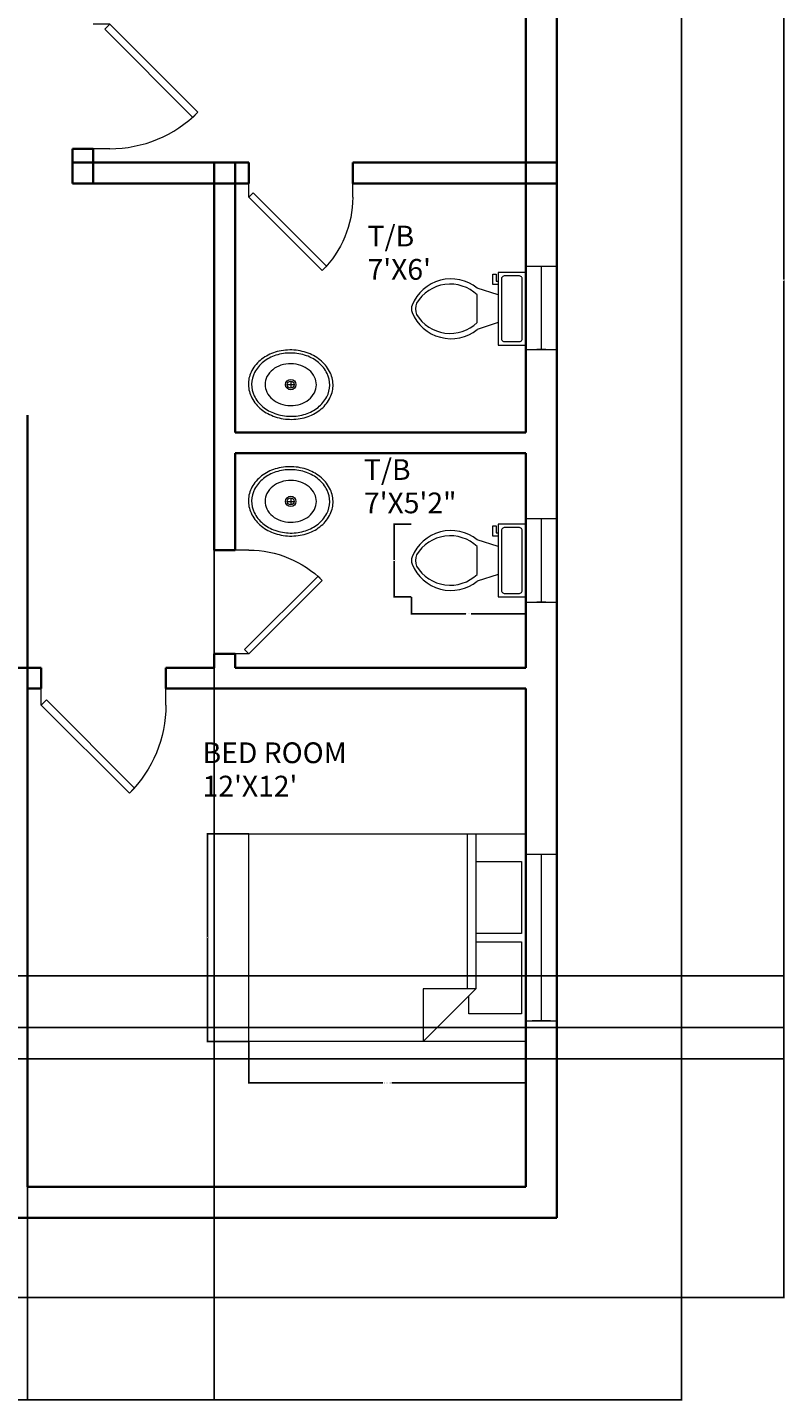
# Model space of a CAD drawing. Units: inches. Extents: x 450 to 1026, y 542 to 1190.
# Tile 7 of 11: x 807 to 1025, y 542 to 939. Entities that reach past the tile are written whole.
import ezdxf

# ---------------------------------------------------------------- set-up
doc = ezdxf.new("R2010")
doc.units = ezdxf.units.IN
doc.header["$MEASUREMENT"] = 0
for name, color, linetype, lineweight in [('A-ANNO-DIMS', 2, 'Continuous', 18), ('A-AREA-IDEN', 7, 'Continuous', 18), ('A-DOOR', 4, 'Continuous', 18), ('A-FLOR-FIXT', 9, 'Continuous', 18), ('A-FURN', 8, 'Continuous', 18), ('A-GLAZ', 4, 'Continuous', 18), ('A-WALL', 7, 'Continuous', 35), ('C-PROP', 7, 'Continuous', 25)]:
    doc.layers.add(name, color=color, linetype=linetype, lineweight=lineweight)
doc.styles.get("Standard").update_dxf_attribs({"font": 'arial.ttf'})
doc.dimstyles.get("Standard").update_dxf_attribs({"dimtxt": 0.18, "dimasz": 0.18, "dimexe": 0.18, "dimexo": 0.0625, "dimgap": 0.09, "dimtad": 0, "dimtih": 1, "dimtoh": 1, "dimdec": 4, "dimzin": 0, "dimdsep": 46, "dimtxsty": 'Standard', "dimcen": 0.09, "dimadec": 0, "dimazin": 0, "dimtfac": 1, "dimtdec": 4, "dimtofl": 0, "dimtmove": 0, "dimatfit": 3, "dimfxl": 1, "dimtolj": 1, "dimtzin": 0, "dimarcsym": 0})

# ---------------------------------------------------------------- blocks, each defined once
blk = doc.blocks.new('*U4')
for p, q in [((0, 0), (0, -100)), ((750, 0), (750, -100))]:
    blk.add_line(p, q)
blk.add_lwpolyline([(0, 0), (530.3, 530.3), (561.3, 499.4), (30.9, -30.9)], close=True)
blk.add_arc((0, 0), 750, 0, 45)
blk = doc.blocks.new('*U3')
for p, q in [((0, 100), (0, 0)), ((900, 100), (900, 0)), ((0, 50), (900, 50))]:
    blk.add_line(p, q)
blk = doc.blocks.new('Bed - Queen')
for p, q in [((0, -80.00003), (0, 0)), ((0, 0), (59.99999, 0)), ((59.99999, 0), (59.99999, -80.00003)), ((7.99999, -1.2), (28.79998, -1.2)), ((7.99999, -14.4), (7.99999, -1.2)), ((28.79998, -1.2), (28.79998, -14.4)), ((31.19999, -1.2), (51.99999, -1.2)), ((31.19999, -14.4), (31.19999, -1.2)), ((51.99999, -1.2), (51.99999, -16.4)), ((0, -14.4), (44.8, -14.4)), ((59.99999, -29.6), (44.8, -14.4)), ((44.8, -14.4), (44.8, -29.6)), ((44.8, -16.8), (0, -16.8)), ((51.99999, -16.4), (46.79936, -16.4)), ((44.8, -29.6), (59.99999, -29.6)), ((59.99999, -80.00003), (0, -80.00003))]:
    blk.add_line(p, q)
blk = doc.blocks.new('Toilet - top')
for p, q in [((9.5, -6), (9.5, -2)), ((-10, -8.5), (-8, -8.5)), ((-10, -9.5), (-10, -8.5)), ((-7, -9.5), (-10, -9.5)), ((-8, -8.5), (-8, -8)), ((-7, -8), (-7, -9.5)), ((-4, -8), (-6, -14)), ((4, -8), (6, -14)), ((4, -14), (-4, -14))]:
    blk.add_line(p, q)
blk.add_lwpolyline([(10.5, -8), (10.5, 0), (-10.5, 0), (-10.5, -8)], close=True)
for points in [[(-9.5, -2), (-9.5, -6)], [(8.5, -1), (-8.5, -1)], [(-8.5, -7), (8.5, -7)]]:
    blk.add_lwpolyline(points)
for centre, radius, start, end in [((-8.62, -1.88), 0.884, 81.8699, 188.1301), ((8.62, -1.88), 0.884, 351.8699, 98.1301), ((-8.62, -6.12), 0.884, 171.8699, 278.1301), ((8.62, -6.12), 0.884, 261.8699, 8.1301), ((3.52, -21.58), 12.17, 141.4691, 247.9714), ((4.2, -21.82), 11.33, 136.3677, 238.9468), ((-3.52, -21.58), 12.17, 292.0284, 38.5307), ((-4.2, -21.82), 11.33, 301.053, 43.6321), ((0, -27.88), 4, 245.7318, 294.2682), ((0, -29), 4, 254.8605, 285.1395)]:
    blk.add_arc(centre, radius, start, end)
blk = doc.blocks.new('Sink - Oval top')
for p, q in [((-1, 0), (1, 0)), ((0, 1), (0, -1))]:
    blk.add_line(p, q)
for points in [[(-12.23, 0.39, 0.117634), (-11.46, -3.36, 0.104469), (-8.88, -6.8, 0.090016), (-5.08, -9.07, 0.08192), (-0.32, -10.02, 0.08192), (4.49, -9.38, 0.090016), (8.42, -7.36, 0.104469), (11.22, -4.09, 0.117634), (12.23, -0.39, 0.117634), (11.46, 3.36, 0.104469), (8.88, 6.8, 0.090016), (5.08, 9.07, 0.08192), (0.32, 10.02, 0.08192), (-4.49, 9.38, 0.090016), (-8.42, 7.36, 0.104469), (-11.22, 4.09, 0.117634)], [(-11.29, 0.16, 0.118622), (-10.52, -3.25, 0.104678), (-8.07, -6.36, 0.089562), (-4.54, -8.37, 0.081185), (-0.13, -9.15, 0.081185), (4.3, -8.49, 0.089562), (7.89, -6.58, 0.104678), (10.42, -3.55, 0.118622), (11.29, -0.16, 0.118622), (10.52, 3.25, 0.104678), (8.07, 6.36, 0.089562), (4.54, 8.37, 0.081185), (0.13, 9.15, 0.081185), (-4.3, 8.49, 0.089562), (-7.89, 6.58, 0.104678), (-10.42, 3.55, 0.118622)], [(-7.42, 0.08, 0.118283), (-6.91, -2.17, 0.104607), (-5.29, -4.21, 0.089718), (-2.97, -5.53, 0.081436), (-0.07, -6.04, 0.081436), (2.84, -5.59, 0.089718), (5.2, -4.33, 0.104607), (6.86, -2.32, 0.118283), (7.42, -0.08, 0.118283), (6.91, 2.17, 0.104607), (5.29, 4.21, 0.089718), (2.97, 5.53, 0.081436), (0.07, 6.04, 0.081436), (-2.84, 5.59, 0.089718), (-5.2, 4.33, 0.104607), (-6.86, 2.32, 0.118283)]]:
    blk.add_lwpolyline(points, format="xyb", close=True)
for radius in [1.5, 1]:
    blk.add_circle((0, 0), radius)
blk = doc.blocks.new('WIN-FRAME-48IN')
for p, q in [((9, 48), (0, 48)), ((9, 0), (9, 48)), ((0, 0), (9, 0))]:
    blk.add_line(p, q)
blk = doc.blocks.new('WIN-FRAME-24IN')
for p, q in [((9, 24), (0, 24)), ((0, 24), (0, 0)), ((0, 0), (9, 0))]:
    blk.add_line(p, q)
blk = doc.blocks.new('*D23')
at = {"layer": 'A-ANNO-DIMS', "color": 0, "lineweight": -2, "transparency": 16777216}
for p, q in [((870.65, 645.88), (870.65, 633.76)), ((950.65, 645.88), (950.65, 633.76)), ((870.83, 633.94), (909.35, 633.94)), ((950.47, 633.94), (911.95, 633.94))]:
    blk.add_line(p, q, dxfattribs=at)
at = {"layer": 'A-ANNO-DIMS', "color": 0, "transparency": 16777216}
for points in [[(870.83, 633.97), (870.83, 633.91), (870.65, 633.94)], [(950.47, 633.97), (950.47, 633.91), (950.65, 633.94)]]:
    blk.add_solid(points, dxfattribs=at)
at = {"layer": 'Defpoints', "color": 0, "transparency": 16777216}
for p in [(870.65, 645.94), (950.65, 645.94), (950.65, 633.94)]:
    blk.add_point(p, dxfattribs=at)
at = {"layer": 'A-ANNO-DIMS', "color": 0, "transparency": 16777216, "insert": (910.65, 633.94), "char_height": 0.18, "attachment_point": 5}
blk.add_mtext('\\A1;QUEEN BED 80 TYP.', dxfattribs=at)
blk = doc.blocks.new('*D24')
at = {"layer": 'A-ANNO-DIMS', "color": 0, "lineweight": -2, "transparency": 16777216}
for p, q in [((870.59, 705.94), (858.47, 705.94)), ((858.65, 705.76), (858.65, 676.12)), ((858.65, 646.12), (858.65, 675.76)), ((870.59, 645.94), (858.47, 645.94))]:
    blk.add_line(p, q, dxfattribs=at)
at = {"layer": 'A-ANNO-DIMS', "color": 0, "transparency": 16777216}
for points in [[(858.62, 705.76), (858.68, 705.76), (858.65, 705.94)], [(858.62, 646.12), (858.68, 646.12), (858.65, 645.94)]]:
    blk.add_solid(points, dxfattribs=at)
at = {"layer": 'Defpoints', "color": 0, "transparency": 16777216}
for p in [(870.65, 705.94), (858.65, 645.94), (870.65, 645.94)]:
    blk.add_point(p, dxfattribs=at)
at = {"layer": 'A-ANNO-DIMS', "color": 0, "transparency": 16777216, "insert": (858.65, 675.94), "char_height": 0.18, "attachment_point": 5}
blk.add_mtext('\\A1;60 TYP.', dxfattribs=at)
blk = doc.blocks.new('*D31')
at = {"layer": 'A-ANNO-DIMS', "color": 0, "lineweight": -2, "transparency": 16777216}
for p, q in [((917.61, 774.38), (917.61, 769.31)), ((950.65, 774.38), (950.65, 769.31)), ((917.79, 769.49), (933.35, 769.49)), ((950.47, 769.49), (934.9, 769.49))]:
    blk.add_line(p, q, dxfattribs=at)
at = {"layer": 'A-ANNO-DIMS', "color": 0, "transparency": 16777216}
for points in [[(917.79, 769.52), (917.79, 769.46), (917.61, 769.49)], [(950.47, 769.52), (950.47, 769.46), (950.65, 769.49)]]:
    blk.add_solid(points, dxfattribs=at)
at = {"layer": 'Defpoints', "color": 0, "transparency": 16777216}
for p in [(917.61, 774.44), (950.65, 774.44), (950.65, 769.49)]:
    blk.add_point(p, dxfattribs=at)
at = {"layer": 'A-ANNO-DIMS', "color": 0, "transparency": 16777216, "insert": (934.13, 769.49), "char_height": 0.18, "attachment_point": 5}
blk.add_mtext('\\A1;WC 33 TYP.', dxfattribs=at)
blk = doc.blocks.new('*D32')
at = {"layer": 'A-ANNO-DIMS', "color": 0, "lineweight": -2, "transparency": 16777216}
for p, q in [((917.54, 795.44), (912.47, 795.44)), ((912.65, 795.26), (912.65, 785.12)), ((912.65, 774.62), (912.65, 784.76)), ((917.54, 774.44), (912.47, 774.44))]:
    blk.add_line(p, q, dxfattribs=at)
at = {"layer": 'A-ANNO-DIMS', "color": 0, "transparency": 16777216}
for points in [[(912.62, 795.26), (912.68, 795.26), (912.65, 795.44)], [(912.62, 774.62), (912.68, 774.62), (912.65, 774.44)]]:
    blk.add_solid(points, dxfattribs=at)
at = {"layer": 'Defpoints', "color": 0, "transparency": 16777216}
for p in [(917.61, 795.44), (912.65, 774.44), (917.61, 774.44)]:
    blk.add_point(p, dxfattribs=at)
at = {"layer": 'A-ANNO-DIMS', "color": 0, "transparency": 16777216, "insert": (912.65, 784.94), "char_height": 0.18, "attachment_point": 5}
blk.add_mtext('\\A1;21 TYP.', dxfattribs=at)
blk = doc.blocks.new('*D45')
at = {"layer": 'A-ANNO-DIMS', "color": 0, "lineweight": -2, "transparency": 16777216}
for p, q in [((479.65, 571.88), (479.65, 542.16)), ((995.65, 571.88), (995.65, 542.16)), ((479.83, 542.34), (737.36, 542.34)), ((995.47, 542.34), (737.94, 542.34))]:
    blk.add_line(p, q, dxfattribs=at)
at = {"layer": 'A-ANNO-DIMS', "color": 0, "transparency": 16777216}
for points in [[(479.83, 542.37), (479.83, 542.31), (479.65, 542.34)], [(995.47, 542.37), (995.47, 542.31), (995.65, 542.34)]]:
    blk.add_solid(points, dxfattribs=at)
at = {"layer": 'Defpoints', "color": 0, "transparency": 16777216}
for p in [(479.65, 571.94), (995.65, 571.94), (995.65, 542.34)]:
    blk.add_point(p, dxfattribs=at)
at = {"layer": 'A-ANNO-DIMS', "color": 0, "transparency": 16777216, "insert": (737.65, 542.34), "char_height": 0.18, "attachment_point": 5}
blk.add_mtext('\\A1;516', dxfattribs=at)
blk = doc.blocks.new('*D46')
at = {"layer": 'A-ANNO-DIMS', "color": 0, "lineweight": -2, "transparency": 16777216}
for p, q in [((995.71, 1159.94), (1025.43, 1159.94)), ((1025.25, 1159.76), (1025.25, 866.12)), ((1025.25, 572.12), (1025.25, 865.76)), ((995.71, 571.94), (1025.43, 571.94))]:
    blk.add_line(p, q, dxfattribs=at)
at = {"layer": 'A-ANNO-DIMS', "color": 0, "transparency": 16777216}
for points in [[(1025.22, 1159.76), (1025.28, 1159.76), (1025.25, 1159.94)], [(1025.22, 572.12), (1025.28, 572.12), (1025.25, 571.94)]]:
    blk.add_solid(points, dxfattribs=at)
at = {"layer": 'Defpoints', "color": 0, "transparency": 16777216}
for p in [(995.65, 1159.94), (1025.25, 1159.94), (995.65, 571.94)]:
    blk.add_point(p, dxfattribs=at)
at = {"layer": 'A-ANNO-DIMS', "color": 0, "transparency": 16777216, "insert": (1025.25, 865.94), "char_height": 0.18, "attachment_point": 5}
blk.add_mtext('\\A1;588', dxfattribs=at)
blk = doc.blocks.new('*D59')
at = {"layer": 'A-ANNO-DIMS', "color": 0, "lineweight": -2, "transparency": 16777216}
for p, q in [((806.65, 817.88), (806.65, 542.16)), ((860.65, 787.88), (860.65, 542.16)), ((806.83, 542.34), (833.43, 542.34)), ((860.47, 542.34), (833.87, 542.34))]:
    blk.add_line(p, q, dxfattribs=at)
at = {"layer": 'A-ANNO-DIMS', "color": 0, "transparency": 16777216}
for points in [[(806.83, 542.37), (806.83, 542.31), (806.65, 542.34)], [(860.47, 542.37), (860.47, 542.31), (860.65, 542.34)]]:
    blk.add_solid(points, dxfattribs=at)
at = {"layer": 'Defpoints', "color": 0, "transparency": 16777216}
for p in [(806.65, 817.94), (860.65, 787.94), (860.65, 542.34)]:
    blk.add_point(p, dxfattribs=at)
at = {"layer": 'A-ANNO-DIMS', "color": 0, "transparency": 16777216, "insert": (833.65, 542.34), "char_height": 0.18, "attachment_point": 5}
blk.add_mtext('\\A1;54', dxfattribs=at)
blk = doc.blocks.new('*D71')
at = {"layer": 'A-ANNO-DIMS', "color": 0, "lineweight": -2, "transparency": 16777216}
for p, q in [((646.71, 649.94), (1025.43, 649.94)), ((1025.25, 649.76), (1025.25, 645.62)), ((1025.25, 641.12), (1025.25, 645.26)), ((637.71, 640.94), (1025.43, 640.94))]:
    blk.add_line(p, q, dxfattribs=at)
at = {"layer": 'A-ANNO-DIMS', "color": 0, "transparency": 16777216}
for points in [[(1025.22, 649.76), (1025.28, 649.76), (1025.25, 649.94)], [(1025.22, 641.12), (1025.28, 641.12), (1025.25, 640.94)]]:
    blk.add_solid(points, dxfattribs=at)
at = {"layer": 'Defpoints', "color": 0, "transparency": 16777216}
for p in [(646.65, 649.94), (1025.25, 649.94), (637.65, 640.94)]:
    blk.add_point(p, dxfattribs=at)
at = {"layer": 'A-ANNO-DIMS', "color": 0, "transparency": 16777216, "insert": (1025.25, 645.44), "char_height": 0.18, "attachment_point": 5}
blk.add_mtext('\\A1;9', dxfattribs=at)
blk = doc.blocks.new('*D72')
at = {"layer": 'A-ANNO-DIMS', "color": 0, "lineweight": -2, "transparency": 16777216}
for p, q in [((643.71, 664.94), (1025.43, 664.94)), ((1025.25, 664.76), (1025.25, 653.12)), ((1025.25, 641.12), (1025.25, 652.76)), ((637.71, 640.94), (1025.43, 640.94))]:
    blk.add_line(p, q, dxfattribs=at)
at = {"layer": 'A-ANNO-DIMS', "color": 0, "transparency": 16777216}
for points in [[(1025.22, 664.76), (1025.28, 664.76), (1025.25, 664.94)], [(1025.22, 641.12), (1025.28, 641.12), (1025.25, 640.94)]]:
    blk.add_solid(points, dxfattribs=at)
at = {"layer": 'Defpoints', "color": 0, "transparency": 16777216}
for p in [(643.65, 664.94), (1025.25, 664.94), (637.65, 640.94)]:
    blk.add_point(p, dxfattribs=at)
at = {"layer": 'A-ANNO-DIMS', "color": 0, "transparency": 16777216, "insert": (1025.25, 652.94), "char_height": 0.18, "attachment_point": 5}
blk.add_mtext('\\A1;24', dxfattribs=at)

msp = doc.modelspace()

# ---------------------------------------------------------------- linework, layer by layer
at = {"layer": 'A-WALL'}
for p, q in [((950.6513, 1064.9426), (950.6513, 821.9426)), ((959.6513, 1064.9426), (959.6513, 594.9426)), ((819.6513, 893.9426), (819.6513, 903.9426)), ((825.6513, 903.9426), (819.6513, 903.9426)), ((825.6513, 893.9426), (825.6513, 903.9426)), ((819.6513, 899.9426), (870.6513, 899.9426)), ((860.6513, 899.9426), (860.6513, 787.9426)), ((866.6513, 899.9426), (866.6513, 821.9426)), ((870.6513, 899.9426), (870.6513, 893.9426)), ((900.6513, 893.9426), (900.6513, 899.9426)), ((900.6513, 899.9426), (959.6513, 899.9426)), ((819.6513, 893.9426), (870.6513, 893.9426)), ((900.6513, 893.9426), (959.6513, 893.9426)), ((806.6513, 826.9426), (806.6513, 603.9426)), ((866.6513, 821.9426), (950.6513, 821.9426)), ((866.6513, 815.9426), (950.6513, 815.9426)), ((866.6513, 815.9426), (866.6513, 787.9426)), ((950.6513, 815.9426), (950.6513, 753.9426)), ((860.6513, 787.9426), (866.6513, 787.9426)), ((866.6513, 757.9426), (860.6513, 757.9426)), ((860.6513, 757.9426), (860.6513, 753.9426)), ((866.6513, 757.9426), (866.6513, 753.9426)), ((801.6513, 753.9426), (810.6513, 753.9426)), ((810.6513, 753.9426), (810.6513, 747.9426)), ((846.6513, 753.9426), (860.6513, 753.9426)), ((846.6513, 747.9426), (846.6513, 753.9426)), ((846.6513, 753.9426), (860.6513, 753.9426)), ((866.6513, 753.9426), (950.6513, 753.9426)), ((806.6513, 747.9426), (810.6513, 747.9426)), ((846.6513, 747.9426), (950.6513, 747.9426)), ((950.6513, 747.9426), (950.6513, 603.9426)), ((806.6513, 603.9426), (950.6513, 603.9426)), ((797.6513, 594.9426), (959.6513, 594.9426))]:
    msp.add_line(p, q, dxfattribs=at)
at = {"layer": 'C-PROP'}
for p in [(995.6513, 1159.9426), (479.6513, 571.9426)]:
    msp.add_line(p, (995.6513, 571.9426), dxfattribs=at)

# ---------------------------------------------------------------- block references
at = {"layer": 'A-DOOR'}
for p, xscale, yscale, zscale, rotation in [((830.4513, 939.9426), 0.048, 0.048, 0.048, 270), ((870.6513, 889.9426), -0.0400000000000003, 0.0400000000000003, 0.0400000000000003, 180), ((870.6513, 757.9426), -0.04, 0.04, 0.04, 270), ((810.6513, 743.1426), -0.048, 0.048, 0.048, 180)]:
    msp.add_blockref('*U4', p, dxfattribs=dict(at, xscale=xscale, yscale=yscale, zscale=zscale, rotation=rotation))
at = {"layer": 'A-FLOR-FIXT', "rotation": 270}
for p in [(950.6513, 857.6905), (950.6513, 784.9426)]:
    msp.add_blockref('Toilet - top', p, dxfattribs=at)
at = {"layer": 'A-FLOR-FIXT'}
for p in [(882.7314, 835.7608), (882.7314, 802.0312)]:
    msp.add_blockref('Sink - Oval top', p, dxfattribs=at)
at = {"layer": 'A-FURN', "rotation": 270.0000000000108}
msp.add_blockref('Bed - Queen', (950.6513, 705.9426), dxfattribs=at)
at = {"layer": 'A-GLAZ', "rotation": 180}
for p in [(959.6517, 869.9421), (959.6517, 796.9421)]:
    msp.add_blockref('WIN-FRAME-24IN', p, dxfattribs=at)
at = {"layer": 'A-GLAZ', "rotation": 270}
for p, xscale, yscale, zscale in [((953.818, 869.9426), 0.0266666666666667, 0.0266666666666667, 0.0266666666666667), ((953.818, 796.9426), 0.0266666666666667, 0.0266666666666667, 0.0266666666666667), ((952.4847, 699.9426), 0.0533333333333333, 0.0533333333333333, 0.0533333333333333)]:
    msp.add_blockref('*U3', p, dxfattribs=dict(at, xscale=xscale, yscale=yscale, zscale=zscale))
at = {"layer": 'A-GLAZ'}
msp.add_blockref('WIN-FRAME-48IN', (950.651, 651.943), dxfattribs=at)

# ---------------------------------------------------------------- texts
at = {"layer": 'A-AREA-IDEN'}
for s, p in [('T/B', (904.9386, 875.7115)), ("7'X6'", (904.9386, 866.0731)), ('T/B', (903.8918, 808.2213)), ('7\'X5\'2"', (903.8918, 798.5828)), ('BED ROOM', (857.2607, 726.3718)), ("12'X12'", (857.2607, 716.7334))]:
    msp.add_text(s, height=6, dxfattribs=at).set_placement(p)

# ---------------------------------------------------------------- dimensions: what is measured, and where the dimension line sits
at = {"layer": 'A-ANNO-DIMS'}
for base, p1, p2, picture, middle in [((1025.2513, 1159.9426), (995.6513, 571.9426), (995.6513, 1159.9426), '*D46', (1025.2513, 865.9426)), ((1025.2513, 664.9426), (637.6513, 640.9426), (643.6513, 664.9426), '*D72', (1025.2513, 652.9426)), ((1025.2513, 649.9426), (637.6513, 640.9426), (646.6513, 649.9426), '*D71', (1025.2513, 645.4426))]:
    dim = msp.add_linear_dim(base=base, p1=p1, p2=p2, angle=90, dimstyle='Standard', override={"dimdec": 0, "dimlfac": 1, "dimrnd": 0, "dimzin": 0, "dimdsep": 46, "dimlunit": 2}, dxfattribs=at)
    dim.commit()
    dim.dimension.update_dxf_attribs({"geometry": picture, "text_midpoint": middle})
for base, p1, p2, picture, middle in [((860.6513, 542.3426), (806.6513, 817.9426), (860.6513, 787.9426), '*D59', (833.6513, 542.3426)), ((995.6513, 542.3426), (479.6513, 571.9426), (995.6513, 571.9426), '*D45', (737.6513, 542.3426))]:
    dim = msp.add_linear_dim(base=base, p1=p1, p2=p2, dimstyle='Standard', override={"dimdec": 0, "dimlfac": 1, "dimrnd": 0, "dimzin": 0, "dimdsep": 46, "dimlunit": 2}, dxfattribs=at)
    dim.commit()
    dim.dimension.update_dxf_attribs({"geometry": picture, "text_midpoint": middle})
for base, p1, p2, angle, text, picture, middle in [((912.6482, 774.4426), (917.6051, 795.4426), (917.6051, 774.4426), 270, '<> TYP.', '*D32', (912.6482, 784.9426)), ((858.6513, 645.9426), (870.6513, 705.9426), (870.6513, 645.9426), 270, '<> TYP.', '*D24', (858.6513, 675.9426)), ((950.6513, 633.9426), (870.6513, 645.9426), (950.6513, 645.9426), 0, 'QUEEN BED <> TYP.', '*D23', (910.6513, 633.9426))]:
    dim = msp.add_linear_dim(base=base, p1=p1, p2=p2, angle=angle, text=text, dimstyle='Standard', override={"dimdec": 0, "dimlfac": 1, "dimrnd": 0, "dimzin": 0, "dimdsep": 46, "dimlunit": 2}, dxfattribs=at)
    dim.commit()
    dim.dimension.update_dxf_attribs({"geometry": picture, "text_midpoint": middle})
dim = msp.add_linear_dim(base=(950.6513, 769.4856), p1=(917.6051, 774.4426), p2=(950.6513, 774.4426), text='WC <> TYP.', dimstyle='Standard', override={"dimdec": 0, "dimlfac": 1, "dimrnd": 0, "dimzin": 0, "dimdsep": 46, "dimlunit": 2}, dxfattribs=at)
dim.commit()
dim.dimension.update_dxf_attribs({"geometry": '*D31', "text_midpoint": (934.1282, 769.4856)})

doc.saveas('drawing.dxf')
